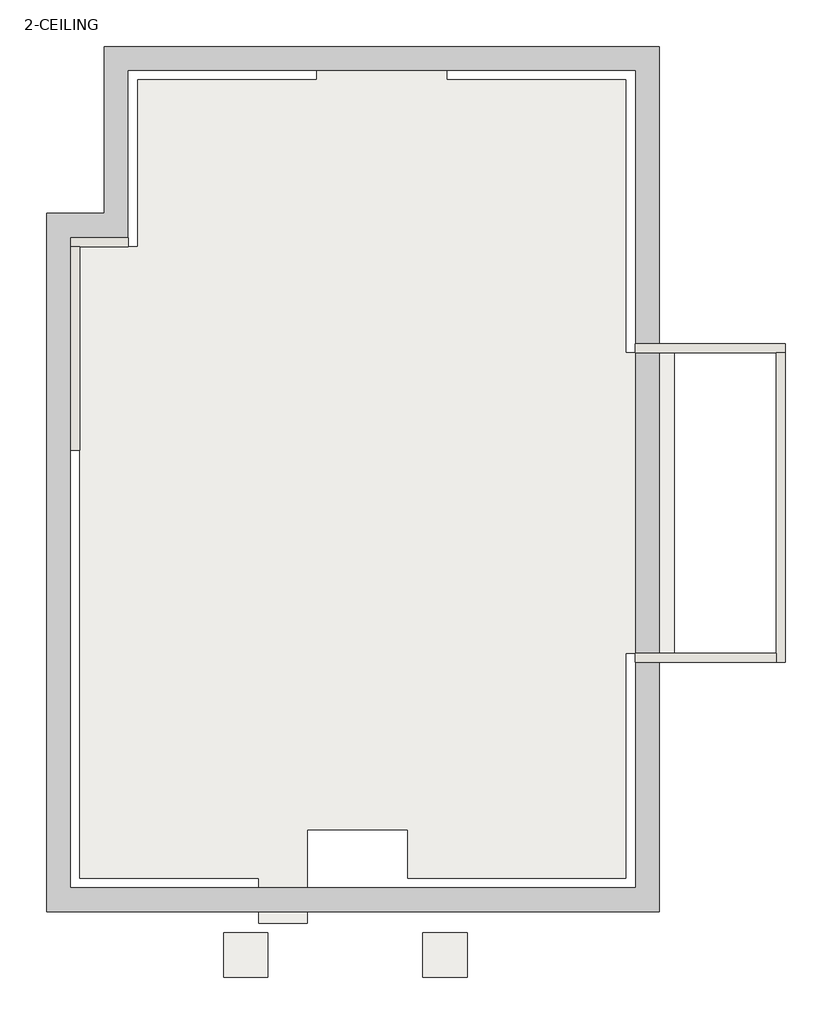
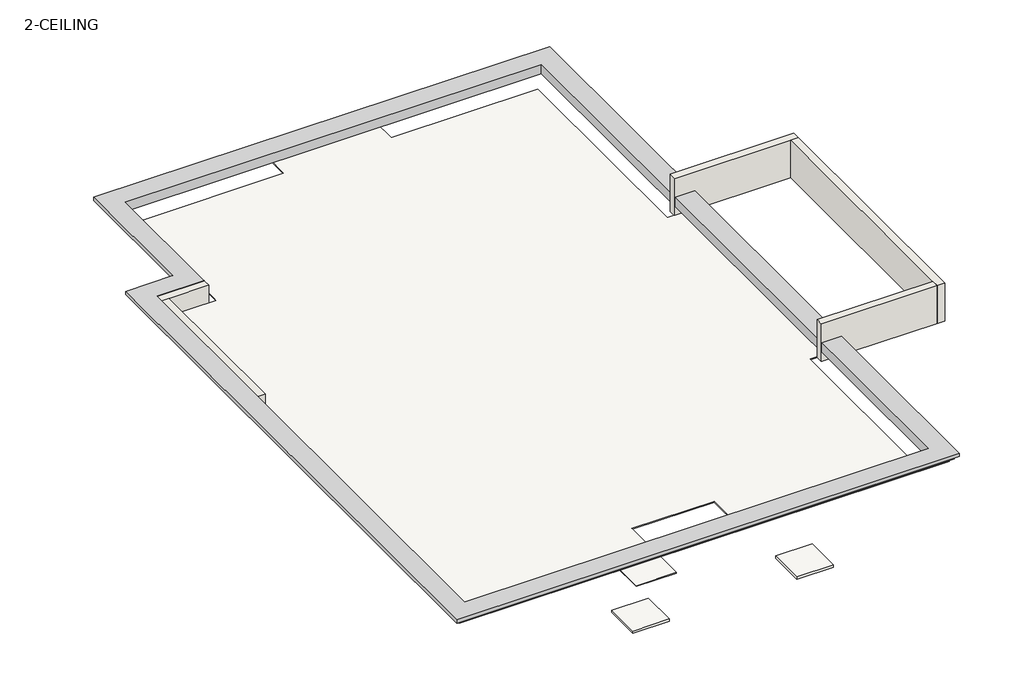
# One storey: 5 walls, 2 slabs, 1 covering, 1 furniture element.
"""IFC4 building model written with IfcOpenShell, lengths in millimetres."""

from ifc_helpers import new_model, si_unit, frame, origin, place, context, project, spatial, polyline, outline, extrude, faceted_brep, transform, mapped, element, save
from components import casework_2_casework_2_b6b509d5

model = new_model("IFC4")

# Units and contexts
model_context = context("Model", 3, world=origin())
ifc_project = project(units=[si_unit("LENGTHUNIT", "METRE", prefix="MILLI")], contexts=[model_context])

# Site, building, storey
site = spatial("IfcSite", under=ifc_project)
building = spatial("IfcBuilding", under=site)
storey = spatial("IfcBuildingStorey", under=building, Name="2-CEILING", Elevation=3450.0)

# Covering
placement = place(None, origin())
element("IfcCovering", 1, ObjectType="Plain", at=placement, inside=storey, context=model_context, shape_type="SweptSolid", body=[
    extrude(outline(polyline([(-36.7953966, 8865.8070837), (-36.7953966, 9690.8070837), (3188.2046034, 9690.8070837), (3188.2046034, 8865.8070837), (7613.2046034, 8865.8070837), (7613.2046034, 4965.8070837), (7613.2046034, 2340.8070837), (7613.2046034, 2115.8070837), (8813.2046034, 2115.8070837), (8813.2046034, -5309.1929163), (7613.2046034, -5309.1929163), (7613.2046034, -10871.6929163), (2213.2046034, -10871.6929163), (2213.2046034, -9671.6929163), (-261.7953966, -9671.6929163), (-261.7953966, -11984.1929163), (-1461.7953966, -11984.1929163), (-1461.7953966, -10871.6929163), (-5886.7953966, -10871.6929163), (-5886.7953966, 4740.8070837), (-4461.7953966, 4740.8070837), (-4461.7953966, 8865.8070837), (-36.7953966, 8865.8070837)])), frame((0.0, 0.0, 3450.0), z_axis=(0.0, 0.0, 1.0), x_axis=(1.0, 0.0, 0.0)), (0.0, 0.0, 1.0), 27.0),
])

# Furniture
casework_2_casework_2_shape = casework_2_casework_2_b6b509d5(model_context)
element("IfcFurniture", 2, ObjectType="Casework 2 : Casework 2", at=placement, inside=storey, context=model_context, shape_type="MappedRepresentation", body=[
    mapped(casework_2_casework_2_shape, transform((0.0, 0.0, 0.0), x_axis=(1.0, 0.0, 0.0), y_axis=(0.0, 1.0, 0.0), z_axis=(0.0, 0.0, 1.0))),
])

# Slabs
element("IfcSlab", 3, ObjectType="75mm", at=placement, inside=storey, context=model_context, shape_type="SweptSolid", body=[
    extrude(outline(polyline([(-1236.7953966, -12224.1929163), (-1236.7953966, -13324.1929163), (-2336.7953966, -13324.1929163), (-2336.7953966, -12224.1929163), (-1236.7953966, -12224.1929163)])), frame((0.0, 0.0, 3075.0), z_axis=(0.0, 0.0, 1.0), x_axis=(1.0, 0.0, 0.0)), (0.0, 0.0, 1.0), 75.0),
])
element("IfcSlab", 4, ObjectType="75mm", at=placement, inside=storey, context=model_context, shape_type="SweptSolid", body=[
    extrude(outline(polyline([(3693.2046034, -12224.1929163), (3693.2046034, -13324.1929163), (2593.2046034, -13324.1929163), (2593.2046034, -12224.1929163), (3693.2046034, -12224.1929163)])), frame((0.0, 0.0, 3075.0), z_axis=(0.0, 0.0, 1.0), x_axis=(1.0, 0.0, 0.0)), (0.0, 0.0, 1.0), 75.0),
])

# Walls
element("IfcWall", 5, ObjectType="225 wall", at=placement, inside=storey, context=model_context, shape_type="SweptSolid", body=[
    extrude(outline(polyline([(-5886.7953966, 4740.8070837), (-5886.7953966, -284.1929163), (-6111.7953966, -284.1929163), (-6111.7953966, 4740.8070837), (-5886.7953966, 4740.8070837)])), frame((0.0, 0.0, 3450.0), z_axis=(0.0, 0.0, 1.0), x_axis=(1.0, 0.0, 0.0)), (0.0, 0.0, 1.0), 592.0),
])
element("IfcWall", 6, ObjectType="225 wall", at=placement, inside=storey, context=model_context, shape_type="Brep", body=[
    faceted_brep([(-4686.7953966, 4965.8070837, 3450.0), (-6111.7953966, 4965.8070837, 3450.0), (-6111.7953966, 4965.8070837, 4042.0), (-4686.7953966, 4965.8070837, 4042.0), (-4686.7953966, 4740.8070837, 3450.0), (-4686.7953966, 4740.8070837, 4042.0), (-5886.7953966, 4740.8070837, 4042.0), (-6111.7953966, 4740.8070837, 4042.0), (-6111.7953966, 4740.8070837, 3450.0), (-5886.7953966, 4740.8070837, 3450.0)], [[[0, 1, 2, 3]], [[4, 5, 6, 7, 8, 9]], [[1, 0, 4, 9, 8]], [[2, 1, 8, 7]], [[3, 2, 7, 6, 5]], [[0, 3, 5, 4]]]),
])
element("IfcWall", 7, ObjectType="225 wall", at=placement, inside=storey, context=model_context, shape_type="Brep", body=[
    faceted_brep([(7838.2046034, 2115.8070837, 3450.0), (11325.7046034, 2115.8070837, 3450.0), (11550.7046034, 2115.8070837, 3450.0), (11550.7046034, 2115.8070837, 4650.0), (11325.7046034, 2115.8070837, 4650.0), (7838.2046034, 2115.8070837, 4650.0), (7838.2046034, 2340.8070837, 3450.0), (7838.2046034, 2340.8070837, 4650.0), (11550.7046034, 2340.8070837, 4650.0), (11550.7046034, 2340.8070837, 3450.0)], [[[0, 1, 2, 3, 4, 5]], [[6, 7, 8, 9]], [[2, 1, 0, 6, 9]], [[5, 4, 3, 8, 7]], [[3, 2, 9, 8]], [[0, 5, 7, 6]]]),
])
element("IfcWall", 8, ObjectType="225 wall", at=placement, inside=storey, context=model_context, shape_type="Brep", body=[
    faceted_brep([(11325.7046034, 2115.8070837, 3450.0), (11325.7046034, -5309.1929163, 3450.0), (11325.7046034, -5534.1929163, 3450.0), (11325.7046034, -5534.1929163, 4650.0), (11325.7046034, -5309.1929163, 4650.0), (11325.7046034, 2115.8070837, 4650.0), (11550.7046034, 2115.8070837, 3450.0), (11550.7046034, 2115.8070837, 4650.0), (11550.7046034, -5534.1929163, 4650.0), (11550.7046034, -5534.1929163, 3450.0)], [[[0, 1, 2, 3, 4, 5]], [[6, 7, 8, 9]], [[2, 1, 0, 6, 9]], [[5, 4, 3, 8, 7]], [[0, 5, 7, 6]], [[3, 2, 9, 8]]]),
])
element("IfcWall", 9, ObjectType="225 wall", at=placement, inside=storey, context=model_context, shape_type="Brep", body=[
    faceted_brep([(11325.7046034, -5309.1929163, 3450.0), (7838.2046034, -5309.1929163, 3450.0), (7838.2046034, -5309.1929163, 4050.0), (7838.2046034, -5309.1929163, 4650.0), (11325.7046034, -5309.1929163, 4650.0), (11325.7046034, -5534.1929163, 3450.0), (11325.7046034, -5534.1929163, 4650.0), (7838.2046034, -5534.1929163, 4650.0), (7838.2046034, -5534.1929163, 3450.0)], [[[0, 1, 2, 3, 4]], [[5, 6, 7, 8]], [[1, 0, 5, 8]], [[4, 3, 7, 6]], [[0, 4, 6, 5]], [[3, 2, 1, 8, 7]]]),
])

save(model, "model.ifc")

# Revit data of these elements
# Type "Plain"
#   built-in parameter 1002203 = 1 (stored number, unit not read)
#   built-in parameter 1002202 = 1 (stored number, unit not read)
#   Layers, outside or top first: 15 mm "Metal Stud Layer" (function 1); 12 mm "Gypsum Wall Board" (function 1)
# Type "75mm"
#   Function = 0
#   Layers, outside or top first: 75 mm no material (function 1)
# Type "225 wall"
#   Layers, outside or top first: 225 mm "Concrete, Cast In Situ" (function 1)
# Element 1 (IfcCovering, "Plain")
#   Height Offset From Level = 0 mm
#   Phase Created = New Construction
#   Materials on its faces: "Gypsum Wall Board", "Metal Stud Layer"
# Element 2 (IfcFurniture, "Casework 2 : Casework 2")
#   Phase Created = New Construction
# Elements 3, 4 (IfcSlab, "75mm")
#   Height Offset From Level = -300 mm
#   Phase Created = New Construction
#   Materials on its faces: "Default Floor"
# Elements 5, 6 (IfcWall, "225 wall")
#   Top Offset = -8 mm
#   Base Offset = 0 mm
#   wall height = 592 mm
#   Phase Created = New Construction
#   Base Constraint = 2-CEILING
#   Top Constraint = 3-ROOF
#   Materials on its faces: "Concrete, Cast In Situ"
# Elements 7, 8, 9 (IfcWall, "225 wall")
#   Top Offset = 600 mm
#   Base Offset = 0 mm
#   wall height = 1200 mm
#   Phase Created = New Construction
#   Base Constraint = 2-CEILING
#   Top Constraint = 3-ROOF
#   Materials on its faces: "Concrete, Cast In Situ"
# Materials
#   "Metal Stud Layer": class "Metal", colour RGB 127 127 127, transparency 0, Description = "Light gauge steel framing, thermal air layer", Cost = 0
#   "Gypsum Wall Board": class "Generic", colour RGB 249 249 249, transparency 0, Description = "Gypsum Wall Board", Cost = 0
#   "Concrete, Cast In Situ": class "Concrete", colour RGB 191 178 173, transparency 0, Description = "physical material", Cost = 0
#   "Default Floor": colour RGB 127 127 127, transparency 0, Cost = 0
